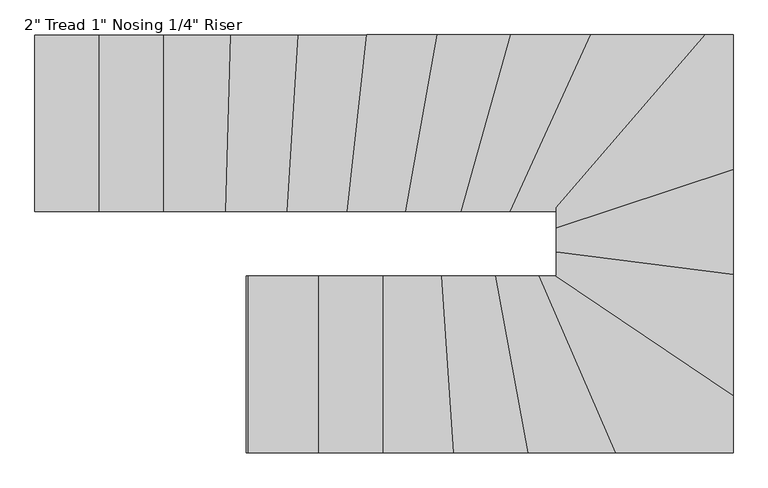
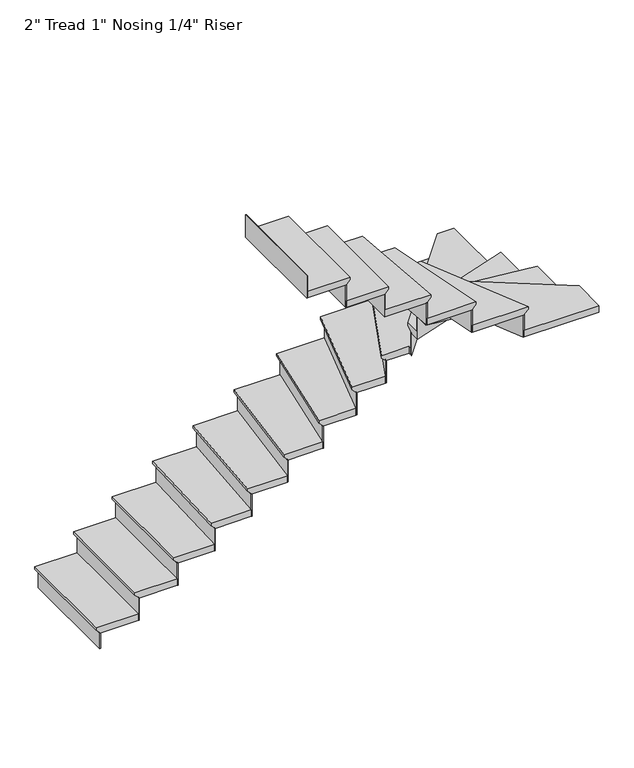
"""IFC4 building model written with IfcOpenShell, lengths in millimetres: stair flight geometry."""

from ifc_helpers import new_model, si_unit, origin, place, context, project, spatial, faceted_brep, source, transform, mapped, element, save


def stair_flight_d882c53c(model_context):
    return source(origin(), model_context, "Body", "Brep", [
        faceted_brep([(-1746.1022736, 2143.0258877, 150.2833333), (-1746.1022736, 2143.0258877, 169.3333333), (-1746.1022736, 2909.8869757, 169.3333333), (-1746.1022736, 2909.8869757, 150.2833333), (-1720.7022736, 2143.0258877, 124.8833333), (-1720.7022736, 2909.8869757, 124.8833333), (-1441.3022736, 2143.0258877, 169.3333333), (-1441.3022736, 2909.8869757, 169.3333333), (-1720.7022736, 2909.8869757, 118.5333333), (-1441.3022736, 2909.8869757, 118.5333333), (-1441.3022736, 2143.0258877, 118.5333333), (-1720.7022736, 2143.0258877, 118.5333333)], [[[0, 1, 2, 3]], [[4, 0, 3, 5]], [[2, 1, 6, 7]], [[8, 9, 10, 11]], [[2, 7, 9, 8, 5, 3]], [[8, 11, 4, 5]], [[6, 1, 0, 4, 11, 10]], [[7, 6, 10, 9]]]),
        faceted_brep([(-1720.7022736, 2143.0258877, 118.5333333), (-1720.7022736, 2143.0258877, 0.0), (-1714.3522736, 2143.0258877, 0.0), (-1714.3522736, 2143.0258877, 118.5333333), (-1720.7022736, 2909.8869757, 118.5333333), (-1714.3522736, 2909.8869757, 118.5333333), (-1714.3522736, 2909.8869757, 0.0), (-1720.7022736, 2909.8869757, 0.0)], [[[0, 1, 2, 3]], [[4, 5, 6, 7]], [[1, 0, 4, 7]], [[2, 1, 7, 6]], [[3, 2, 6, 5]], [[0, 3, 5, 4]]]),
        faceted_brep([(-1441.3022736, 2143.0258877, 287.8666667), (-1441.3022736, 2143.0258877, 118.5333333), (-1434.9522736, 2143.0258877, 118.5333333), (-1434.9522736, 2143.0258877, 287.8666667), (-1441.3022736, 2909.8869757, 287.8666667), (-1434.9522736, 2909.8869757, 287.8666667), (-1434.9522736, 2909.8869757, 118.5333333), (-1441.3022736, 2909.8869757, 118.5333333)], [[[0, 1, 2, 3]], [[4, 5, 6, 7]], [[1, 0, 4, 7]], [[2, 1, 7, 6]], [[3, 2, 6, 5]], [[0, 3, 5, 4]]]),
        faceted_brep([(-1466.7022736, 2909.8869757, 338.6666667), (-1466.7022736, 2143.0258877, 338.6666667), (-1161.9022736, 2143.0258877, 338.6666667), (-1161.9022736, 2909.8869757, 338.6666667), (-1441.3022736, 2909.8869757, 287.8666667), (-1161.9022736, 2909.8869757, 287.8666667), (-1161.9022736, 2143.0258877, 287.8666667), (-1441.3022736, 2143.0258877, 287.8666667), (-1441.3022736, 2909.8869757, 294.2166667), (-1466.7022736, 2909.8869757, 319.6166667), (-1441.3022736, 2143.0258877, 294.2166667), (-1466.7022736, 2143.0258877, 319.6166667)], [[[0, 1, 2, 3]], [[4, 5, 6, 7]], [[0, 3, 5, 4, 8, 9]], [[4, 7, 10, 8]], [[2, 1, 11, 10, 7, 6]], [[3, 2, 6, 5]], [[11, 1, 0, 9]], [[10, 11, 9, 8]]]),
        faceted_brep([(-1161.9022736, 2143.0258877, 457.2), (-1161.9022736, 2143.0258877, 287.8666667), (-1155.5522736, 2143.0258877, 287.8666667), (-1155.5522736, 2143.0258877, 457.2), (-1161.9022736, 2909.8869757, 457.2), (-1155.5522736, 2909.8869757, 457.2), (-1155.5522736, 2909.8869757, 287.8666667), (-1161.9022736, 2909.8869757, 287.8666667)], [[[0, 1, 2, 3]], [[4, 5, 6, 7]], [[1, 0, 4, 7]], [[2, 1, 7, 6]], [[3, 2, 6, 5]], [[0, 3, 5, 4]]]),
        faceted_brep([(-1187.3022736, 2909.8869757, 508.0), (-1187.3022736, 2143.0258877, 508.0), (-892.8998869, 2143.0258877, 508.0), (-872.0859521, 2909.8869757, 508.0), (-1161.9022736, 2909.8869757, 457.2), (-872.0859521, 2909.8869757, 457.2), (-892.8998869, 2143.0258877, 457.2), (-1161.9022736, 2143.0258877, 457.2), (-1161.9022736, 2909.8869757, 463.55), (-1187.3022736, 2909.8869757, 488.95), (-1161.9022736, 2143.0258877, 463.55), (-1187.3022736, 2143.0258877, 488.95)], [[[0, 1, 2, 3]], [[4, 5, 6, 7]], [[0, 3, 5, 4, 8, 9]], [[4, 7, 10, 8]], [[2, 1, 11, 10, 7, 6]], [[3, 2, 6, 5]], [[11, 1, 0, 9]], [[10, 11, 9, 8]]]),
        faceted_brep([(-892.8998869, 2143.0258877, 626.5333333), (-892.8998869, 2143.0258877, 457.2), (-886.5475484, 2143.0258877, 457.2), (-886.5475484, 2143.0258877, 626.5333333), (-872.0859521, 2909.8869757, 626.5333333), (-865.7336136, 2909.8869757, 626.5333333), (-865.7336136, 2909.8869757, 457.2), (-872.0859521, 2909.8869757, 457.2)], [[[0, 1, 2, 3]], [[4, 5, 6, 7]], [[1, 0, 4, 7]], [[2, 1, 7, 6]], [[3, 2, 6, 5]], [[0, 3, 5, 4]]]),
        faceted_brep([(-897.4953062, 2909.8869757, 677.3333333), (-918.3092409, 2143.0258877, 677.3333333), (-626.9430097, 2143.0258877, 677.3333333), (-579.1630295, 2909.8869757, 677.3333333), (-872.0859521, 2909.8869757, 626.5333333), (-579.1630295, 2909.8869757, 626.5333333), (-626.9430097, 2143.0258877, 626.5333333), (-892.8998869, 2143.0258877, 626.5333333), (-872.0859521, 2909.8869757, 632.8833333), (-897.4953062, 2909.8869757, 658.2833333), (-892.8998869, 2143.0258877, 632.8833333), (-918.3092409, 2143.0258877, 658.2833333)], [[[0, 1, 2, 3]], [[4, 5, 6, 7]], [[0, 3, 5, 4, 8, 9]], [[4, 7, 10, 8]], [[2, 1, 11, 10, 7, 6]], [[3, 2, 6, 5]], [[11, 1, 0, 9]], [[10, 11, 9, 8]]]),
        faceted_brep([(-626.9430097, 2143.0258877, 795.8666667), (-626.9430097, 2143.0258877, 626.5333333), (-620.5806962, 2143.0258877, 626.5333333), (-620.5806962, 2143.0258877, 795.8666667), (-579.1630295, 2909.8869757, 795.8666667), (-572.800716, 2909.8869757, 795.8666667), (-572.800716, 2909.8869757, 626.5333333), (-579.1630295, 2909.8869757, 626.5333333)], [[[0, 1, 2, 3]], [[4, 5, 6, 7]], [[1, 0, 4, 7]], [[2, 1, 7, 6]], [[3, 2, 6, 5]], [[0, 3, 5, 4]]]),
        faceted_brep([(-604.6122835, 2909.8869757, 846.6666667), (-652.3922637, 2143.0258877, 846.6666667), (-365.599383, 2143.0258877, 846.6666667), (-281.5005992, 2909.8869757, 846.6666667), (-579.1630295, 2909.8869757, 795.8666667), (-281.5005992, 2909.8869757, 795.8666667), (-365.599383, 2143.0258877, 795.8666667), (-626.9430097, 2143.0258877, 795.8666667), (-579.1630295, 2909.8869757, 802.2166667), (-604.6122835, 2909.8869757, 827.6166667), (-626.9430097, 2143.0258877, 802.2166667), (-652.3922637, 2143.0258877, 827.6166667)], [[[0, 1, 2, 3]], [[4, 5, 6, 7]], [[0, 3, 5, 4, 8, 9]], [[4, 7, 10, 8]], [[2, 1, 11, 10, 7, 6]], [[3, 2, 6, 5]], [[11, 1, 0, 9]], [[10, 11, 9, 8]]]),
        faceted_brep([(-365.599383, 2143.0258877, 965.2), (-365.599383, 2143.0258877, 795.8666667), (-359.2113124, 2143.0258877, 795.8666667), (-359.2113124, 2143.0258877, 965.2), (-281.5005992, 2909.8869757, 965.2), (-275.1125286, 2909.8869757, 965.2), (-275.1125286, 2909.8869757, 795.8666667), (-281.5005992, 2909.8869757, 795.8666667)], [[[0, 1, 2, 3]], [[4, 5, 6, 7]], [[1, 0, 4, 7]], [[2, 1, 7, 6]], [[3, 2, 6, 5]], [[0, 3, 5, 4]]]),
        faceted_brep([(-307.0528817, 2909.8869757, 1016.0), (-391.1516655, 2143.0258877, 1016.0), (-111.7364007, 2143.0258877, 1016.0), (23.9205797, 2909.8869757, 1016.0), (-281.5005992, 2909.8869757, 965.2), (23.9205797, 2909.8869757, 965.2), (-111.7364007, 2143.0258877, 965.2), (-365.599383, 2143.0258877, 965.2), (-281.5005992, 2909.8869757, 971.55), (-307.0528817, 2909.8869757, 996.95), (-365.599383, 2143.0258877, 971.55), (-391.1516655, 2143.0258877, 996.95)], [[[0, 1, 2, 3]], [[4, 5, 6, 7]], [[0, 3, 5, 4, 8, 9]], [[4, 7, 10, 8]], [[2, 1, 11, 10, 7, 6]], [[3, 2, 6, 5]], [[11, 1, 0, 9]], [[10, 11, 9, 8]]]),
        faceted_brep([(-111.7364007, 2143.0258877, 1134.5333333), (-111.7364007, 2143.0258877, 965.2), (-105.28781, 2143.0258877, 965.2), (-105.28781, 2143.0258877, 1134.5333333), (23.9205797, 2909.8869757, 1134.5333333), (30.3691704, 2909.8869757, 1134.5333333), (30.3691704, 2909.8869757, 965.2), (23.9205797, 2909.8869757, 965.2)], [[[0, 1, 2, 3]], [[4, 5, 6, 7]], [[1, 0, 4, 7]], [[2, 1, 7, 6]], [[3, 2, 6, 5]], [[0, 3, 5, 4]]]),
        faceted_brep([(-1.8737833, 2909.8869757, 1185.3333333), (-137.5307638, 2143.0258877, 1185.3333333), (128.7770359, 2143.0258877, 1185.3333333), (343.3699156, 2909.8869757, 1185.3333333), (23.9205797, 2909.8869757, 1134.5333333), (343.3699156, 2909.8869757, 1134.5333333), (128.7770359, 2143.0258877, 1134.5333333), (-111.7364007, 2143.0258877, 1134.5333333), (23.9205797, 2909.8869757, 1140.8833333), (-1.8737833, 2909.8869757, 1166.2833333), (-111.7364007, 2143.0258877, 1140.8833333), (-137.5307638, 2143.0258877, 1166.2833333)], [[[0, 1, 2, 3]], [[4, 5, 6, 7]], [[0, 3, 5, 4, 8, 9]], [[4, 7, 10, 8]], [[2, 1, 11, 10, 7, 6]], [[3, 2, 6, 5]], [[11, 1, 0, 9]], [[10, 11, 9, 8]]]),
        faceted_brep([(128.7770359, 2143.0258877, 1303.8666667), (128.7770359, 2143.0258877, 1134.5333333), (135.3709732, 2143.0258877, 1134.5333333), (135.3709732, 2143.0258877, 1303.8666667), (343.3699156, 2909.8869757, 1303.8666667), (349.963853, 2909.8869757, 1303.8666667), (349.963853, 2909.8869757, 1134.5333333), (343.3699156, 2909.8869757, 1134.5333333)], [[[0, 1, 2, 3]], [[4, 5, 6, 7]], [[1, 0, 4, 7]], [[2, 1, 7, 6]], [[3, 2, 6, 5]], [[0, 3, 5, 4]]]),
        faceted_brep([(316.9941663, 2909.8869757, 1354.6666667), (102.4012866, 2143.0258877, 1354.6666667), (341.7285577, 2143.0258877, 1354.6666667), (692.3241693, 2909.8869757, 1354.6666667), (343.3699156, 2909.8869757, 1303.8666667), (692.3241693, 2909.8869757, 1303.8666667), (341.7285577, 2143.0258877, 1303.8666667), (128.7770359, 2143.0258877, 1303.8666667), (343.3699156, 2909.8869757, 1310.2166667), (316.9941663, 2909.8869757, 1335.6166667), (128.7770359, 2143.0258877, 1310.2166667), (102.4012866, 2143.0258877, 1335.6166667)], [[[0, 1, 2, 3]], [[4, 5, 6, 7]], [[0, 3, 5, 4, 8, 9]], [[4, 7, 10, 8]], [[3, 2, 6, 5]], [[11, 1, 0, 9]], [[10, 11, 9, 8]], [[2, 1, 11, 10, 7, 6]]]),
        faceted_brep([(341.7285577, 2143.0258877, 1473.2), (341.7285577, 2143.0258877, 1303.8666667), (348.710717, 2143.0258877, 1303.8666667), (348.710717, 2143.0258877, 1473.2), (692.3241693, 2909.8869757, 1473.2), (699.3063286, 2909.8869757, 1473.2), (699.3063286, 2909.8869757, 1303.8666667), (692.3241693, 2909.8869757, 1303.8666667)], [[[0, 1, 2, 3]], [[4, 5, 6, 7]], [[1, 0, 4, 7]], [[2, 1, 7, 6]], [[3, 2, 6, 5]], [[0, 3, 5, 4]]]),
        faceted_brep([(664.3955322, 2909.8869757, 1524.0), (313.7999206, 2143.0258877, 1524.0), (513.6752551, 2143.0258877, 1524.0), (513.6752551, 2121.6326599, 1524.0), (1192.4089945, 2909.8869757, 1524.0), (692.3241693, 2909.8869757, 1473.2), (1192.4089945, 2909.8869757, 1473.2), (513.6752551, 2121.6326599, 1473.2), (513.6752551, 2143.0258877, 1473.2), (341.7285577, 2143.0258877, 1473.2), (692.3241693, 2909.8869757, 1479.55), (664.3955322, 2909.8869757, 1504.95), (341.7285577, 2143.0258877, 1479.55), (313.7999206, 2143.0258877, 1504.95)], [[[0, 1, 2, 3, 4]], [[5, 6, 7, 8, 9]], [[0, 4, 6, 5, 10, 11]], [[5, 9, 12, 10]], [[2, 1, 13, 12, 9, 8]], [[4, 3, 7, 6]], [[13, 1, 0, 11]], [[12, 13, 11, 10]], [[3, 2, 8, 7]]]),
        faceted_brep([(513.6752551, 2121.6326599, 1642.5333333), (513.6752551, 2121.6326599, 1473.2), (513.6752551, 2111.9008682, 1473.2), (513.6752551, 2111.9008682, 1642.5333333), (1192.4089945, 2909.8869757, 1642.5333333), (1200.7886446, 2909.8869757, 1642.5333333), (1200.7886446, 2909.8869757, 1473.2), (1192.4089945, 2909.8869757, 1473.2)], [[[0, 1, 2, 3]], [[4, 5, 6, 7]], [[1, 0, 4, 7]], [[2, 1, 7, 6]], [[3, 2, 6, 5]], [[0, 3, 5, 4]]]),
        faceted_brep([(1280.536343, 2299.2693046, 1693.3333333), (1280.536343, 2909.8869757, 1693.3333333), (1158.890394, 2909.8869757, 1693.3333333), (513.6752551, 2160.5598268, 1693.3333333), (513.6752551, 2045.8758981, 1693.3333333), (1280.536343, 2909.8869757, 1642.5333333), (1280.536343, 2299.2693046, 1642.5333333), (513.6752551, 2045.8758981, 1642.5333333), (513.6752551, 2121.6326599, 1642.5333333), (1192.4089945, 2909.8869757, 1642.5333333), (513.6752551, 2121.6326599, 1648.8833333), (1192.4089945, 2909.8869757, 1648.8833333), (513.6752551, 2160.5598268, 1674.2833333), (1158.890394, 2909.8869757, 1674.2833333)], [[[0, 1, 2, 3, 4]], [[5, 6, 7, 8, 9]], [[1, 0, 6, 5]], [[9, 8, 10, 11]], [[4, 3, 12, 10, 8, 7]], [[0, 4, 7, 6]], [[12, 3, 2, 13]], [[10, 12, 13, 11]], [[2, 1, 5, 9, 11, 13]]]),
        faceted_brep([(513.6752551, 2045.8758981, 1811.8666667), (513.6752551, 2045.8758981, 1642.5333333), (513.6752551, 2039.1882189, 1642.5333333), (513.6752551, 2039.1882189, 1811.8666667), (1280.536343, 2299.2693046, 1811.8666667), (1280.536343, 2292.5816253, 1811.8666667), (1280.536343, 2292.5816253, 1642.5333333), (1280.536343, 2299.2693046, 1642.5333333)], [[[0, 1, 2, 3]], [[4, 5, 6, 7]], [[1, 0, 4, 7]], [[2, 1, 7, 6]], [[3, 2, 6, 5]], [[0, 3, 5, 4]]]),
        faceted_brep([(1280.536343, 2326.0200216, 1862.6666667), (513.6752551, 2072.6266151, 1862.6666667), (513.6752551, 1941.6327755, 1862.6666667), (1280.536343, 1844.4445022, 1862.6666667), (1280.536343, 2299.2693046, 1811.8666667), (1280.536343, 1844.4445022, 1811.8666667), (513.6752551, 1941.6327755, 1811.8666667), (513.6752551, 2045.8758981, 1811.8666667), (1280.536343, 2299.2693046, 1818.2166667), (1280.536343, 2326.0200216, 1843.6166667), (513.6752551, 2045.8758981, 1818.2166667), (513.6752551, 2072.6266151, 1843.6166667)], [[[0, 1, 2, 3]], [[4, 5, 6, 7]], [[0, 3, 5, 4, 8, 9]], [[4, 7, 10, 8]], [[2, 1, 11, 10, 7, 6]], [[3, 2, 6, 5]], [[11, 1, 0, 9]], [[10, 11, 9, 8]]]),
        faceted_brep([(513.6752551, 1941.6327755, 1981.2), (513.6752551, 1941.6327755, 1811.8666667), (513.6752551, 1935.2319824, 1811.8666667), (513.6752551, 1935.2319824, 1981.2), (1280.536343, 1844.4445022, 1981.2), (1280.536343, 1838.0437091, 1981.2), (1280.536343, 1838.0437091, 1811.8666667), (1280.536343, 1844.4445022, 1811.8666667)], [[[0, 1, 2, 3]], [[4, 5, 6, 7]], [[1, 0, 4, 7]], [[2, 1, 7, 6]], [[3, 2, 6, 5]], [[0, 3, 5, 4]]]),
        faceted_brep([(1280.536343, 1870.0476746, 2032.0), (513.6752551, 1967.2359478, 2032.0), (513.6752551, 1863.6258877, 2032.0), (464.7938966, 1863.6258877, 2032.0), (1280.536343, 1312.504238, 2032.0), (1280.536343, 1844.4445022, 1981.2), (1280.536343, 1312.504238, 1981.2), (464.7938966, 1863.6258877, 1981.2), (513.6752551, 1863.6258877, 1981.2), (513.6752551, 1941.6327755, 1981.2), (1280.536343, 1844.4445022, 1987.55), (1280.536343, 1870.0476746, 2012.95), (513.6752551, 1941.6327755, 1987.55), (513.6752551, 1967.2359478, 2012.95)], [[[0, 1, 2, 3, 4]], [[5, 6, 7, 8, 9]], [[0, 4, 6, 5, 10, 11]], [[5, 9, 12, 10]], [[2, 1, 13, 12, 9, 8]], [[4, 3, 7, 6]], [[13, 1, 0, 11]], [[12, 13, 11, 10]], [[3, 2, 8, 7]]]),
        faceted_brep([(464.7938966, 1863.6258877, 2150.5333333), (464.7938966, 1863.6258877, 1981.2), (453.4509362, 1863.6258877, 1981.2), (453.4509362, 1863.6258877, 2150.5333333), (1280.536343, 1312.504238, 2150.5333333), (1280.536343, 1304.8408498, 2150.5333333), (1280.536343, 1304.8408498, 1981.2), (1280.536343, 1312.504238, 1981.2)], [[[0, 1, 2, 3]], [[4, 5, 6, 7]], [[1, 0, 4, 7]], [[2, 1, 7, 6]], [[3, 2, 6, 5]], [[0, 3, 5, 4]]]),
        faceted_brep([(741.4901836, 1096.7647998, 2201.3333333), (1280.536343, 1096.7647998, 2201.3333333), (1280.536343, 1343.1577909, 2201.3333333), (510.1657383, 1863.6258877, 2201.3333333), (410.5008095, 1863.6258877, 2201.3333333), (1280.536343, 1096.7647998, 2150.5333333), (741.4901836, 1096.7647998, 2150.5333333), (410.5008095, 1863.6258877, 2150.5333333), (464.7938966, 1863.6258877, 2150.5333333), (1280.536343, 1312.504238, 2150.5333333), (464.7938966, 1863.6258877, 2156.8833333), (1280.536343, 1312.504238, 2156.8833333), (510.1657383, 1863.6258877, 2182.2833333), (1280.536343, 1343.1577909, 2182.2833333)], [[[0, 1, 2, 3, 4]], [[5, 6, 7, 8, 9]], [[1, 0, 6, 5]], [[9, 8, 10, 11]], [[4, 3, 12, 10, 8, 7]], [[0, 4, 7, 6]], [[12, 3, 2, 13]], [[10, 12, 13, 11]], [[2, 1, 5, 9, 11, 13]]]),
        faceted_brep([(410.5008095, 1863.6258877, 2319.8666667), (410.5008095, 1863.6258877, 2150.5333333), (403.5845773, 1863.6258877, 2150.5333333), (403.5845773, 1863.6258877, 2319.8666667), (741.4901836, 1096.7647998, 2319.8666667), (734.5739514, 1096.7647998, 2319.8666667), (734.5739514, 1096.7647998, 2150.5333333), (741.4901836, 1096.7647998, 2150.5333333)], [[[0, 1, 2, 3]], [[4, 5, 6, 7]], [[1, 0, 4, 7]], [[2, 1, 7, 6]], [[3, 2, 6, 5]], [[0, 3, 5, 4]]]),
        faceted_brep([(769.1551123, 1096.7647998, 2370.6666667), (438.1657383, 1863.6258877, 2370.6666667), (223.2979515, 1863.6258877, 2370.6666667), (365.5040004, 1096.7647998, 2370.6666667), (741.4901836, 1096.7647998, 2319.8666667), (365.5040004, 1096.7647998, 2319.8666667), (223.2979515, 1863.6258877, 2319.8666667), (410.5008095, 1863.6258877, 2319.8666667), (741.4901836, 1096.7647998, 2326.2166667), (769.1551123, 1096.7647998, 2351.6166667), (410.5008095, 1863.6258877, 2326.2166667), (438.1657383, 1863.6258877, 2351.6166667)], [[[0, 1, 2, 3]], [[4, 5, 6, 7]], [[0, 3, 5, 4, 8, 9]], [[4, 7, 10, 8]], [[2, 1, 11, 10, 7, 6]], [[3, 2, 6, 5]], [[11, 1, 0, 9]], [[10, 11, 9, 8]]]),
        faceted_brep([(223.2979515, 1863.6258877, 2489.2), (223.2979515, 1863.6258877, 2319.8666667), (216.8396935, 1863.6258877, 2319.8666667), (216.8396935, 1863.6258877, 2489.2), (365.5040004, 1096.7647998, 2489.2), (359.0457424, 1096.7647998, 2489.2), (359.0457424, 1096.7647998, 2319.8666667), (365.5040004, 1096.7647998, 2319.8666667)], [[[0, 1, 2, 3]], [[4, 5, 6, 7]], [[1, 0, 4, 7]], [[2, 1, 7, 6]], [[3, 2, 6, 5]], [[0, 3, 5, 4]]]),
        faceted_brep([(391.3370325, 1096.7647998, 2540.0), (249.1309836, 1863.6258877, 2540.0), (-10.9124526, 1863.6258877, 2540.0), (41.6612272, 1096.7647998, 2540.0), (365.5040004, 1096.7647998, 2489.2), (41.6612272, 1096.7647998, 2489.2), (-10.9124526, 1863.6258877, 2489.2), (223.2979515, 1863.6258877, 2489.2), (365.5040004, 1096.7647998, 2495.55), (391.3370325, 1096.7647998, 2520.95), (223.2979515, 1863.6258877, 2495.55), (249.1309836, 1863.6258877, 2520.95)], [[[0, 1, 2, 3]], [[4, 5, 6, 7]], [[0, 3, 5, 4, 8, 9]], [[4, 7, 10, 8]], [[2, 1, 11, 10, 7, 6]], [[3, 2, 6, 5]], [[11, 1, 0, 9]], [[10, 11, 9, 8]]]),
        faceted_brep([(-10.9124526, 1863.6258877, 2658.5333333), (-10.9124526, 1863.6258877, 2489.2), (-17.2773578, 1863.6258877, 2489.2), (-17.2773578, 1863.6258877, 2658.5333333), (41.6612272, 1096.7647998, 2658.5333333), (35.296322, 1096.7647998, 2658.5333333), (35.296322, 1096.7647998, 2489.2), (41.6612272, 1096.7647998, 2489.2)], [[[0, 1, 2, 3]], [[4, 5, 6, 7]], [[1, 0, 4, 7]], [[2, 1, 7, 6]], [[3, 2, 6, 5]], [[0, 3, 5, 4]]]),
        faceted_brep([(67.1208479, 1096.7647998, 2709.3333333), (14.5471682, 1863.6258877, 2709.3333333), (-263.9659919, 1863.6258877, 2709.3333333), (-263.9659919, 1096.7647998, 2709.3333333), (41.6612272, 1096.7647998, 2658.5333333), (-263.9659919, 1096.7647998, 2658.5333333), (-263.9659919, 1863.6258877, 2658.5333333), (-10.9124526, 1863.6258877, 2658.5333333), (41.6612272, 1096.7647998, 2664.8833333), (67.1208479, 1096.7647998, 2690.2833333), (-10.9124526, 1863.6258877, 2664.8833333), (14.5471682, 1863.6258877, 2690.2833333)], [[[0, 1, 2, 3]], [[4, 5, 6, 7]], [[0, 3, 5, 4, 8, 9]], [[4, 7, 10, 8]], [[2, 1, 11, 10, 7, 6]], [[3, 2, 6, 5]], [[11, 1, 0, 9]], [[10, 11, 9, 8]]]),
        faceted_brep([(-263.9659919, 1863.6258877, 2827.8666667), (-263.9659919, 1863.6258877, 2658.5333333), (-270.3159919, 1863.6258877, 2658.5333333), (-270.3159919, 1863.6258877, 2827.8666667), (-263.9659919, 1096.7647998, 2827.8666667), (-270.3159919, 1096.7647998, 2827.8666667), (-270.3159919, 1096.7647998, 2658.5333333), (-263.9659919, 1096.7647998, 2658.5333333)], [[[0, 1, 2, 3]], [[4, 5, 6, 7]], [[1, 0, 4, 7]], [[2, 1, 7, 6]], [[3, 2, 6, 5]], [[0, 3, 5, 4]]]),
        faceted_brep([(-238.5659919, 1096.7647998, 2878.6666667), (-238.5659919, 1863.6258877, 2878.6666667), (-543.3659919, 1863.6258877, 2878.6666667), (-543.3659919, 1096.7647998, 2878.6666667), (-263.9659919, 1096.7647998, 2827.8666667), (-543.3659919, 1096.7647998, 2827.8666667), (-543.3659919, 1863.6258877, 2827.8666667), (-263.9659919, 1863.6258877, 2827.8666667), (-263.9659919, 1096.7647998, 2834.2166667), (-238.5659919, 1096.7647998, 2859.6166667), (-263.9659919, 1863.6258877, 2834.2166667), (-238.5659919, 1863.6258877, 2859.6166667)], [[[0, 1, 2, 3]], [[4, 5, 6, 7]], [[0, 3, 5, 4, 8, 9]], [[4, 7, 10, 8]], [[2, 1, 11, 10, 7, 6]], [[3, 2, 6, 5]], [[11, 1, 0, 9]], [[10, 11, 9, 8]]]),
        faceted_brep([(-543.3659919, 1863.6258877, 2997.2), (-543.3659919, 1863.6258877, 2827.8666667), (-549.7159919, 1863.6258877, 2827.8666667), (-549.7159919, 1863.6258877, 2997.2), (-543.3659919, 1096.7647998, 2997.2), (-549.7159919, 1096.7647998, 2997.2), (-549.7159919, 1096.7647998, 2827.8666667), (-543.3659919, 1096.7647998, 2827.8666667)], [[[0, 1, 2, 3]], [[4, 5, 6, 7]], [[1, 0, 4, 7]], [[2, 1, 7, 6]], [[3, 2, 6, 5]], [[0, 3, 5, 4]]]),
        faceted_brep([(-822.7659919, 1863.6258877, 3166.5333333), (-822.7659919, 1863.6258877, 2997.2), (-829.1159919, 1863.6258877, 2997.2), (-829.1159919, 1863.6258877, 3166.5333333), (-822.7659919, 1096.7647998, 3166.5333333), (-829.1159919, 1096.7647998, 3166.5333333), (-829.1159919, 1096.7647998, 2997.2), (-822.7659919, 1096.7647998, 2997.2)], [[[0, 1, 2, 3]], [[4, 5, 6, 7]], [[1, 0, 4, 7]], [[2, 1, 7, 6]], [[3, 2, 6, 5]], [[0, 3, 5, 4]]]),
        faceted_brep([(-517.9659919, 1096.7647998, 3048.0), (-517.9659919, 1863.6258877, 3048.0), (-822.7659919, 1863.6258877, 3048.0), (-822.7659919, 1096.7647998, 3048.0), (-543.3659919, 1096.7647998, 2997.2), (-822.7659919, 1096.7647998, 2997.2), (-822.7659919, 1863.6258877, 2997.2), (-543.3659919, 1863.6258877, 2997.2), (-543.3659919, 1096.7647998, 3003.55), (-517.9659919, 1096.7647998, 3028.95), (-543.3659919, 1863.6258877, 3003.55), (-517.9659919, 1863.6258877, 3028.95)], [[[0, 1, 2, 3]], [[4, 5, 6, 7]], [[0, 3, 5, 4, 8, 9]], [[4, 7, 10, 8]], [[2, 1, 11, 10, 7, 6]], [[3, 2, 6, 5]], [[11, 1, 0, 9]], [[10, 11, 9, 8]]]),
    ])


if __name__ == "__main__":
    model = new_model("IFC4")
    model_context = context("Model", 3, world=origin())
    ifc_project = project(units=[si_unit("LENGTHUNIT", "METRE", prefix="MILLI")], contexts=[model_context])
    site = spatial("IfcSite", under=ifc_project)
    building = spatial("IfcBuilding", under=site)
    placement = place(None, origin())
    stair_flight_shape = stair_flight_d882c53c(model_context)
    element("IfcStairFlight", 1, ObjectType="2\" Tread 1\" Nosing 1/4\" Riser", at=placement, inside=building, context=model_context, shape_type="MappedRepresentation", body=[
        mapped(stair_flight_shape, transform((0.0, 0.0, 0.0), x_axis=(1.0, 0.0, 0.0), y_axis=(0.0, 1.0, 0.0), z_axis=(0.0, 0.0, 1.0))),
    ])
    save(model, "model.ifc")
